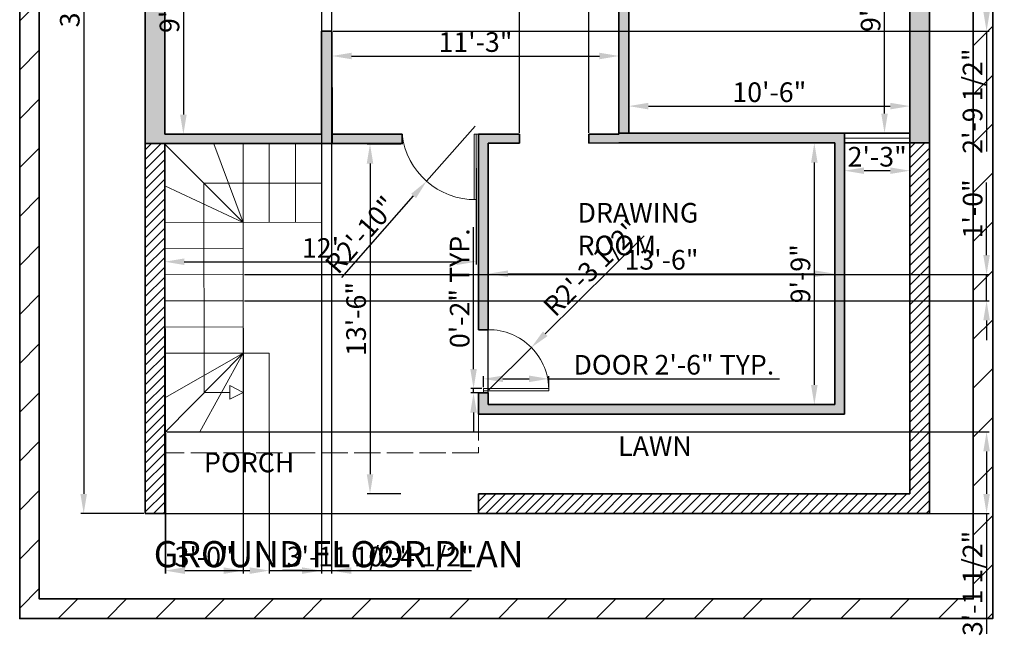
# Model space of a CAD drawing. Units: inches. Extents: x 1130698 to 1131150, y 432269 to 432875.
# Tile 1 of 3: x 1130698 to 1131150, y 432269 to 432551. Entities that reach past the tile are written whole.
import ezdxf

# ---------------------------------------------------------------- set-up
doc = ezdxf.new("R2010")
doc.units = ezdxf.units.IN
doc.linetypes.add('ACAD_ISO02W100', pattern=[15, 12, -3])
for name, color, linetype, lineweight in [('A-ANNO-DIMS', 2, 'Continuous', 18), ('A-ANNO-TEXT', 7, 'Continuous', 25), ('A-ANNO-TTLB', 7, 'Continuous', 35), ('A-AREA-IDEN', 7, 'Continuous', 25), ('A-DOOR', 4, 'Continuous', 18), ('A-FLOR-STRS', 7, 'Continuous', 18), ('A-GLAZ', 4, 'Continuous', 18), ('A-ROOF-OVHD', 8, 'ACAD_ISO02W100', 13), ('A-WALL', 7, 'Continuous', 35)]:
    doc.layers.add(name, color=color, linetype=linetype, lineweight=lineweight)
doc.layers.add('A-ANNO-TTLB-PATT', color=251, linetype='Continuous', lineweight=13, true_color=0x636466)
doc.layers.add('A-WALL-PATT', color=251, linetype='Continuous', lineweight=13, true_color=0x636466)
doc.styles.get("Standard").update_dxf_attribs({"font": 'arial.ttf'})
doc.dimstyles.new('ISO-25', dxfattribs={"dimtxt": 9, "dimasz": 9, "dimexe": 1.25, "dimexo": 0.625, "dimtad": 1, "dimdec": 1, "dimrnd": 9, "dimlunit": 3, "dimtxsty": 'Standard', "dimcen": 2.5, "dimadec": 0, "dimazin": 0, "dimtfac": 1, "dimtdec": 1, "dimtmove": 0, "dimatfit": 3, "dimfxl": 1, "dimarcsym": 0})

# ---------------------------------------------------------------- blocks, each defined once
blk = doc.blocks.new('*D11')
at = {"layer": 'A-ANNO-DIMS', "color": 0, "lineweight": -2, "transparency": 16777216}
for p, q in [((1130977.75, 432499.73), (1130977.75, 432512.76)), ((1130986.75, 432511.51), (1131097.75, 432511.51)), ((1131106.75, 432499.73), (1131106.75, 432512.76))]:
    blk.add_line(p, q, dxfattribs=at)
at = {"layer": 'A-ANNO-DIMS', "color": 0, "transparency": 16777216}
for points in [[(1130986.75, 432513.01), (1130986.75, 432510.01), (1130977.75, 432511.51)], [(1131097.75, 432513.01), (1131097.75, 432510.01), (1131106.75, 432511.51)]]:
    blk.add_solid(points, dxfattribs=at)
at = {"layer": 'Defpoints', "color": 0, "transparency": 16777216}
for p in [(1131106.75, 432511.51), (1130977.75, 432499.11), (1131106.75, 432499.11)]:
    blk.add_point(p, dxfattribs=at)
at = {"layer": 'A-ANNO-DIMS', "color": 0, "transparency": 16777216, "insert": (1131042.25, 432516.73), "char_height": 9, "attachment_point": 5}
blk.add_mtext('10\'-6"', dxfattribs=at)
blk = doc.blocks.new('*D12')
at = {"layer": 'A-ANNO-DIMS', "color": 0, "lineweight": -2, "transparency": 16777216}
for p, q in [((1131106.12, 432619.11), (1131093.87, 432619.11)), ((1131095.12, 432508.11), (1131095.12, 432610.11)), ((1131106.12, 432499.11), (1131093.87, 432499.11))]:
    blk.add_line(p, q, dxfattribs=at)
at = {"layer": 'A-ANNO-DIMS', "color": 0, "transparency": 16777216}
for points in [[(1131093.62, 432610.11), (1131096.62, 432610.11), (1131095.12, 432619.11)], [(1131093.62, 432508.11), (1131096.62, 432508.11), (1131095.12, 432499.11)]]:
    blk.add_solid(points, dxfattribs=at)
at = {"layer": 'Defpoints', "color": 0, "transparency": 16777216}
for p in [(1131095.12, 432619.11), (1131106.75, 432619.11), (1131106.75, 432499.11)]:
    blk.add_point(p, dxfattribs=at)
at = {"layer": 'A-ANNO-DIMS', "color": 0, "transparency": 16777216, "insert": (1131089.9, 432559.11), "char_height": 9, "attachment_point": 5, "rotation": 90}
blk.add_mtext('9\'-9"', dxfattribs=at)
blk = doc.blocks.new('*D13')
at = {"layer": 'A-ANNO-DIMS', "color": 0, "lineweight": -2, "transparency": 16777216}
for p, q in [((1130765.37, 432618.61), (1130774.58, 432618.61)), ((1130773.33, 432609.61), (1130773.33, 432507.61)), ((1130765.37, 432498.61), (1130774.58, 432498.61))]:
    blk.add_line(p, q, dxfattribs=at)
at = {"layer": 'A-ANNO-DIMS', "color": 0, "transparency": 16777216}
for points in [[(1130771.83, 432609.61), (1130774.83, 432609.61), (1130773.33, 432618.61)], [(1130771.83, 432507.61), (1130774.83, 432507.61), (1130773.33, 432498.61)]]:
    blk.add_solid(points, dxfattribs=at)
at = {"layer": 'Defpoints', "color": 0, "transparency": 16777216}
for p in [(1130764.75, 432618.61), (1130764.75, 432498.61), (1130773.33, 432498.61)]:
    blk.add_point(p, dxfattribs=at)
at = {"layer": 'A-ANNO-DIMS', "color": 0, "transparency": 16777216, "insert": (1130768.11, 432558.61), "char_height": 9, "attachment_point": 5, "rotation": 90}
blk.add_mtext('9\'-9"', dxfattribs=at)
blk = doc.blocks.new('*D15')
at = {"layer": 'A-ANNO-DIMS', "color": 0, "lineweight": -2, "transparency": 16777216}
for p, q in [((1130841.53, 432499.23), (1130841.53, 432535.75)), ((1130850.53, 432534.5), (1130964.25, 432534.5)), ((1130973.25, 432499.73), (1130973.25, 432535.75))]:
    blk.add_line(p, q, dxfattribs=at)
at = {"layer": 'A-ANNO-DIMS', "color": 0, "transparency": 16777216}
for points in [[(1130850.53, 432536), (1130850.53, 432533), (1130841.53, 432534.5)], [(1130964.25, 432536), (1130964.25, 432533), (1130973.25, 432534.5)]]:
    blk.add_solid(points, dxfattribs=at)
at = {"layer": 'Defpoints', "color": 0, "transparency": 16777216}
for p in [(1130973.25, 432534.5), (1130841.53, 432498.61), (1130973.25, 432499.11)]:
    blk.add_point(p, dxfattribs=at)
at = {"layer": 'A-ANNO-DIMS', "color": 0, "transparency": 16777216, "insert": (1130907.39, 432539.73), "char_height": 9, "attachment_point": 5}
blk.add_mtext('11\'-3"', dxfattribs=at)
blk = doc.blocks.new('*D16')
at = {"layer": 'A-ANNO-DIMS', "color": 0, "lineweight": -2, "transparency": 16777216}
for p, q in [((1131071.62, 432494.61), (1131061.65, 432494.61)), ((1131062.9, 432485.61), (1131062.9, 432383.61)), ((1131071.62, 432374.61), (1131061.65, 432374.61))]:
    blk.add_line(p, q, dxfattribs=at)
at = {"layer": 'A-ANNO-DIMS', "color": 0, "transparency": 16777216}
for points in [[(1131061.4, 432485.61), (1131064.4, 432485.61), (1131062.9, 432494.61)], [(1131061.4, 432383.61), (1131064.4, 432383.61), (1131062.9, 432374.61)]]:
    blk.add_solid(points, dxfattribs=at)
at = {"layer": 'Defpoints', "color": 0, "transparency": 16777216}
for p in [(1131072.25, 432494.61), (1131062.9, 432374.61), (1131072.25, 432374.61)]:
    blk.add_point(p, dxfattribs=at)
at = {"layer": 'A-ANNO-DIMS', "color": 0, "transparency": 16777216, "insert": (1131057.68, 432434.61), "char_height": 9, "attachment_point": 5, "rotation": 90}
blk.add_mtext('9\'-9"', dxfattribs=at)
blk = doc.blocks.new('*D17')
at = {"layer": 'A-ANNO-DIMS', "color": 0, "lineweight": -2, "transparency": 16777216}
for p, q in [((1130913.25, 432375.23), (1130913.25, 432435.86)), ((1130922.25, 432434.61), (1131063.25, 432434.61)), ((1131072.25, 432375.23), (1131072.25, 432435.86))]:
    blk.add_line(p, q, dxfattribs=at)
at = {"layer": 'A-ANNO-DIMS', "color": 0, "transparency": 16777216}
for points in [[(1130922.25, 432436.11), (1130922.25, 432433.11), (1130913.25, 432434.61)], [(1131063.25, 432436.11), (1131063.25, 432433.11), (1131072.25, 432434.61)]]:
    blk.add_solid(points, dxfattribs=at)
at = {"layer": 'Defpoints', "color": 0, "transparency": 16777216}
for p in [(1131072.25, 432434.61), (1130913.25, 432374.61), (1131072.25, 432374.61)]:
    blk.add_point(p, dxfattribs=at)
at = {"layer": 'A-ANNO-DIMS', "color": 0, "transparency": 16777216, "insert": (1130992.75, 432439.83), "char_height": 9, "attachment_point": 5}
blk.add_mtext('13\'-6"', dxfattribs=at)
blk = doc.blocks.new('*D18')
at = {"layer": 'A-ANNO-DIMS', "color": 0, "lineweight": -2, "transparency": 16777216}
for p, q in [((1130873.07, 432494.11), (1130857.73, 432494.11)), ((1130858.98, 432485.11), (1130858.98, 432342.61)), ((1130873.07, 432333.61), (1130857.73, 432333.61))]:
    blk.add_line(p, q, dxfattribs=at)
at = {"layer": 'A-ANNO-DIMS', "color": 0, "transparency": 16777216}
for points in [[(1130857.48, 432485.11), (1130860.48, 432485.11), (1130858.98, 432494.11)], [(1130857.48, 432342.61), (1130860.48, 432342.61), (1130858.98, 432333.61)]]:
    blk.add_solid(points, dxfattribs=at)
at = {"layer": 'Defpoints', "color": 0, "transparency": 16777216}
for p in [(1130873.7, 432494.11), (1130858.98, 432333.61), (1130873.7, 432333.61)]:
    blk.add_point(p, dxfattribs=at)
at = {"layer": 'A-ANNO-DIMS', "color": 0, "transparency": 16777216, "insert": (1130853.76, 432413.86), "char_height": 9, "attachment_point": 5, "rotation": 90}
blk.add_mtext('13\'-6"', dxfattribs=at)
blk = doc.blocks.new('*D19')
at = {"layer": 'A-ANNO-DIMS', "color": 0, "lineweight": -2, "transparency": 16777216}
for p, q in [((1130764.75, 432493.48), (1130764.75, 432438.87)), ((1130907.75, 432482.98), (1130907.75, 432438.87)), ((1130773.75, 432440.12), (1130898.75, 432440.12))]:
    blk.add_line(p, q, dxfattribs=at)
at = {"layer": 'A-ANNO-DIMS', "color": 0, "transparency": 16777216}
for points in [[(1130773.75, 432441.62), (1130773.75, 432438.62), (1130764.75, 432440.12)], [(1130898.75, 432441.62), (1130898.75, 432438.62), (1130907.75, 432440.12)]]:
    blk.add_solid(points, dxfattribs=at)
at = {"layer": 'Defpoints', "color": 0, "transparency": 16777216}
for p in [(1130764.75, 432494.11), (1130907.75, 432483.61), (1130907.75, 432440.12)]:
    blk.add_point(p, dxfattribs=at)
at = {"layer": 'A-ANNO-DIMS', "color": 0, "transparency": 16777216, "insert": (1130836.25, 432445.26), "char_height": 9, "attachment_point": 5}
blk.add_mtext("12'", dxfattribs=at)
blk = doc.blocks.new('*D21')
at = {"layer": 'A-ANNO-DIMS', "color": 0, "lineweight": -2, "transparency": 16777216}
for p, q in [((1130755.12, 432804.61), (1130726.33, 432804.61)), ((1130727.58, 432795.61), (1130727.58, 432333.61)), ((1130755.12, 432324.61), (1130726.33, 432324.61))]:
    blk.add_line(p, q, dxfattribs=at)
at = {"layer": 'A-ANNO-DIMS', "color": 0, "transparency": 16777216}
for points in [[(1130726.08, 432795.61), (1130729.08, 432795.61), (1130727.58, 432804.61)], [(1130726.08, 432333.61), (1130729.08, 432333.61), (1130727.58, 432324.61)]]:
    blk.add_solid(points, dxfattribs=at)
at = {"layer": 'Defpoints', "color": 0, "transparency": 16777216}
for p in [(1130755.75, 432804.61), (1130727.58, 432324.61), (1130755.75, 432324.61)]:
    blk.add_point(p, dxfattribs=at)
at = {"layer": 'A-ANNO-DIMS', "color": 0, "transparency": 16777216, "insert": (1130722.35, 432564.61), "char_height": 9, "attachment_point": 5, "rotation": 90}
blk.add_mtext('39\'-9"', dxfattribs=at)
blk = doc.blocks.new('*D22')
at = {"layer": 'A-ANNO-DIMS', "color": 0, "lineweight": -2, "transparency": 16777216}
for p, q in [((1131076.75, 432493.98), (1131076.75, 432480.63)), ((1131106.75, 432493.98), (1131106.75, 432480.63)), ((1131097.75, 432481.88), (1131085.75, 432481.88))]:
    blk.add_line(p, q, dxfattribs=at)
at = {"layer": 'A-ANNO-DIMS', "color": 0, "transparency": 16777216}
for points in [[(1131085.75, 432483.38), (1131085.75, 432480.38), (1131076.75, 432481.88)], [(1131097.75, 432483.38), (1131097.75, 432480.38), (1131106.75, 432481.88)]]:
    blk.add_solid(points, dxfattribs=at)
at = {"layer": 'Defpoints', "color": 0, "transparency": 16777216}
for p in [(1131076.75, 432494.61), (1131106.75, 432494.61), (1131076.75, 432481.88)]:
    blk.add_point(p, dxfattribs=at)
at = {"layer": 'A-ANNO-DIMS', "color": 0, "transparency": 16777216, "insert": (1131091.75, 432487.11), "char_height": 9, "attachment_point": 5}
blk.add_mtext('2\'-3"', dxfattribs=at)
blk = doc.blocks.new('DOOR-LEAF-30IN')
for p, q in [((30, 2), (0, 2)), ((0, 2), (0, 1)), ((0, 0), (0, 1)), ((0, 1), (30, 1)), ((30, 1), (30, 2))]:
    blk.add_line(p, q)
blk = doc.blocks.new('*D28')
at = {"layer": 'A-ANNO-DIMS', "color": 0, "lineweight": -2, "transparency": 16777216}
for p, q in [((1130911, 432382.53), (1130911, 432387.65)), ((1130941, 432382.53), (1130941, 432387.65)), ((1130920, 432386.4), (1130932, 432386.4)), ((1130941, 432386.4), (1131046.87, 432386.4))]:
    blk.add_line(p, q, dxfattribs=at)
at = {"layer": 'A-ANNO-DIMS', "color": 0, "transparency": 16777216}
for points in [[(1130920, 432387.9), (1130920, 432384.9), (1130911, 432386.4)], [(1130932, 432387.9), (1130932, 432384.9), (1130941, 432386.4)]]:
    blk.add_solid(points, dxfattribs=at)
at = {"layer": 'Defpoints', "color": 0, "transparency": 16777216}
for p in [(1130941, 432386.4), (1130911, 432381.9), (1130941, 432381.9)]:
    blk.add_point(p, dxfattribs=at)
at = {"layer": 'A-ANNO-DIMS', "color": 0, "transparency": 16777216, "insert": (1130998.43, 432391.69), "char_height": 9, "attachment_point": 5}
blk.add_mtext('DOOR 2\'-6" TYP.', dxfattribs=at)
blk = doc.blocks.new('*D29')
at = {"layer": 'A-ANNO-DIMS', "color": 0, "lineweight": -2, "transparency": 16777216}
for p, q in [((1130906.5, 432390.9), (1130906.5, 432456.01)), ((1130910.37, 432381.9), (1130905.25, 432381.9)), ((1130910.37, 432379.9), (1130905.25, 432379.9)), ((1130906.5, 432379.9), (1130906.5, 432381.9)), ((1130906.5, 432370.9), (1130906.5, 432361.9))]:
    blk.add_line(p, q, dxfattribs=at)
at = {"layer": 'A-ANNO-DIMS', "color": 0, "transparency": 16777216}
for points in [[(1130905, 432390.9), (1130908, 432390.9), (1130906.5, 432381.9)], [(1130905, 432370.9), (1130908, 432370.9), (1130906.5, 432379.9)]]:
    blk.add_solid(points, dxfattribs=at)
at = {"layer": 'Defpoints', "color": 0, "transparency": 16777216}
for p in [(1130906.5, 432381.9), (1130911, 432381.9), (1130911, 432379.9)]:
    blk.add_point(p, dxfattribs=at)
at = {"layer": 'A-ANNO-DIMS', "color": 0, "transparency": 16777216, "insert": (1130901.28, 432427.96), "char_height": 9, "attachment_point": 5, "rotation": 90}
blk.add_mtext('0\'-2" TYP.', dxfattribs=at)
blk = doc.blocks.new('*D32')
at = {"layer": 'A-ANNO-DIMS', "color": 0, "lineweight": -2, "transparency": 16777216}
for p, q in [((1130765.06, 432361.48), (1130765.06, 432297.16)), ((1130812.75, 432361.6), (1130812.75, 432297.16)), ((1130774.06, 432298.41), (1130803.75, 432298.41)), ((1130812.75, 432298.41), (1130874.88, 432298.41))]:
    blk.add_line(p, q, dxfattribs=at)
at = {"layer": 'A-ANNO-DIMS', "color": 0, "transparency": 16777216}
for points in [[(1130774.06, 432299.91), (1130774.06, 432296.91), (1130765.06, 432298.41)], [(1130803.75, 432299.91), (1130803.75, 432296.91), (1130812.75, 432298.41)]]:
    blk.add_solid(points, dxfattribs=at)
at = {"layer": 'Defpoints', "color": 0, "transparency": 16777216}
for p in [(1130765.06, 432362.11), (1130812.75, 432362.22), (1130812.75, 432298.41)]:
    blk.add_point(p, dxfattribs=at)
at = {"layer": 'A-ANNO-DIMS', "color": 0, "transparency": 16777216, "insert": (1130848.31, 432303.69), "char_height": 9, "attachment_point": 5}
blk.add_mtext('3\'-11 1/2"', dxfattribs=at)
blk = doc.blocks.new('*D33')
at = {"layer": 'A-ANNO-DIMS', "color": 0, "lineweight": -2, "transparency": 16777216}
for p, q in [((1131141.95, 432443.19), (1131141.95, 432476.52)), ((1130801.37, 432434.19), (1131143.2, 432434.19)), ((1131141.95, 432422.19), (1131141.95, 432434.19)), ((1130801.37, 432422.19), (1131143.2, 432422.19)), ((1131141.95, 432413.19), (1131141.95, 432404.19))]:
    blk.add_line(p, q, dxfattribs=at)
at = {"layer": 'A-ANNO-DIMS', "color": 0, "transparency": 16777216}
for points in [[(1131140.45, 432443.19), (1131143.45, 432443.19), (1131141.95, 432434.19)], [(1131140.45, 432413.19), (1131143.45, 432413.19), (1131141.95, 432422.19)]]:
    blk.add_solid(points, dxfattribs=at)
at = {"layer": 'Defpoints', "color": 0, "transparency": 16777216}
for p in [(1130800.75, 432434.19), (1131141.95, 432434.19), (1130800.75, 432422.19)]:
    blk.add_point(p, dxfattribs=at)
at = {"layer": 'A-ANNO-DIMS', "color": 0, "transparency": 16777216, "insert": (1131136.73, 432464.36), "char_height": 9, "attachment_point": 5, "rotation": 90}
blk.add_mtext('1\'-0"', dxfattribs=at)
blk = doc.blocks.new('*D34')
at = {"layer": 'A-ANNO-DIMS', "color": 0, "lineweight": -2, "transparency": 16777216}
for p, q in [((1130764.95, 432409.48), (1130764.95, 432297.16)), ((1130800.75, 432409.57), (1130800.75, 432297.16)), ((1130773.95, 432298.41), (1130791.75, 432298.41))]:
    blk.add_line(p, q, dxfattribs=at)
at = {"layer": 'A-ANNO-DIMS', "color": 0, "transparency": 16777216}
for points in [[(1130773.95, 432299.91), (1130773.95, 432296.91), (1130764.95, 432298.41)], [(1130791.75, 432299.91), (1130791.75, 432296.91), (1130800.75, 432298.41)]]:
    blk.add_solid(points, dxfattribs=at)
at = {"layer": 'Defpoints', "color": 0, "transparency": 16777216}
for p in [(1130764.95, 432410.11), (1130800.75, 432410.19), (1130800.75, 432298.41)]:
    blk.add_point(p, dxfattribs=at)
at = {"layer": 'A-ANNO-DIMS', "color": 0, "transparency": 16777216, "insert": (1130782.85, 432303.63), "char_height": 9, "attachment_point": 5}
blk.add_mtext('3\'-0"', dxfattribs=at)
blk = doc.blocks.new('*D35')
at = {"layer": 'A-ANNO-DIMS', "color": 0, "lineweight": -2, "transparency": 16777216}
for p, q in [((1130765.69, 432362.11), (1131143.2, 432362.11)), ((1131141.95, 432353.11), (1131141.95, 432333.61)), ((1130765.37, 432324.61), (1131143.2, 432324.61)), ((1131141.95, 432324.61), (1131141.95, 432269.47))]:
    blk.add_line(p, q, dxfattribs=at)
at = {"layer": 'A-ANNO-DIMS', "color": 0, "transparency": 16777216}
for points in [[(1131140.45, 432353.11), (1131143.45, 432353.11), (1131141.95, 432362.11)], [(1131140.45, 432333.61), (1131143.45, 432333.61), (1131141.95, 432324.61)]]:
    blk.add_solid(points, dxfattribs=at)
at = {"layer": 'Defpoints', "color": 0, "transparency": 16777216}
for p in [(1130765.06, 432362.11), (1130764.75, 432324.61), (1131141.95, 432324.61)]:
    blk.add_point(p, dxfattribs=at)
at = {"layer": 'A-ANNO-DIMS', "color": 0, "transparency": 16777216, "insert": (1131136.66, 432292.54), "char_height": 9, "attachment_point": 5, "rotation": 90}
blk.add_mtext('3\'-1 1/2"', dxfattribs=at)
blk = doc.blocks.new('*D36')
at = {"layer": 'A-ANNO-DIMS', "color": 0, "lineweight": -2, "transparency": 16777216}
for p, q in [((1130841.96, 432579.47), (1131143.2, 432579.47)), ((1131141.95, 432570.47), (1131141.95, 432554.94)), ((1130842.05, 432545.94), (1131143.2, 432545.94)), ((1131141.95, 432545.94), (1131141.95, 432490.64))]:
    blk.add_line(p, q, dxfattribs=at)
at = {"layer": 'A-ANNO-DIMS', "color": 0, "transparency": 16777216}
for points in [[(1131140.45, 432570.47), (1131143.45, 432570.47), (1131141.95, 432579.47)], [(1131140.45, 432554.94), (1131143.45, 432554.94), (1131141.95, 432545.94)]]:
    blk.add_solid(points, dxfattribs=at)
at = {"layer": 'Defpoints', "color": 0, "transparency": 16777216}
for p in [(1130841.34, 432579.47), (1130841.42, 432545.94), (1131141.95, 432545.94)]:
    blk.add_point(p, dxfattribs=at)
at = {"layer": 'A-ANNO-DIMS', "color": 0, "transparency": 16777216, "insert": (1131136.67, 432513.79), "char_height": 9, "attachment_point": 5, "rotation": 90}
blk.add_mtext('2\'-9 1/2"', dxfattribs=at)
blk = doc.blocks.new('*D38')
at = {"layer": 'A-ANNO-DIMS', "color": 0, "lineweight": -2, "transparency": 16777216}
for p, q in [((1130927.61, 432499.23), (1130927.61, 432832.06)), ((1130936.61, 432830.81), (1130950.44, 432830.81)), ((1130959.44, 432499.23), (1130959.44, 432832.06))]:
    blk.add_line(p, q, dxfattribs=at)
at = {"layer": 'A-ANNO-DIMS', "color": 0, "transparency": 16777216}
for points in [[(1130936.61, 432832.31), (1130936.61, 432829.31), (1130927.61, 432830.81)], [(1130950.44, 432832.31), (1130950.44, 432829.31), (1130959.44, 432830.81)]]:
    blk.add_solid(points, dxfattribs=at)
at = {"layer": 'Defpoints', "color": 0, "transparency": 16777216}
for p in [(1130959.44, 432830.81), (1130927.61, 432498.61), (1130959.44, 432498.61)]:
    blk.add_point(p, dxfattribs=at)
at = {"layer": 'A-ANNO-DIMS', "color": 0, "transparency": 16777216, "insert": (1130943.52, 432836.03), "char_height": 9, "attachment_point": 5}
blk.add_mtext('2\'-8"', dxfattribs=at)
blk = doc.blocks.new('*D39')
at = {"layer": 'A-ANNO-DIMS', "color": 0, "lineweight": -2, "transparency": 16777216}
for p, q in [((1130950.44, 432830.81), (1130941.44, 432830.81)), ((1130959.44, 432499.23), (1130959.44, 432832.06)), ((1130959.44, 432830.81), (1130973.25, 432830.81)), ((1130973.25, 432499.73), (1130973.25, 432832.06)), ((1130982.25, 432830.81), (1131015.57, 432830.81))]:
    blk.add_line(p, q, dxfattribs=at)
at = {"layer": 'A-ANNO-DIMS', "color": 0, "transparency": 16777216}
for points in [[(1130950.44, 432832.31), (1130950.44, 432829.31), (1130959.44, 432830.81)], [(1130982.25, 432832.31), (1130982.25, 432829.31), (1130973.25, 432830.81)]]:
    blk.add_solid(points, dxfattribs=at)
at = {"layer": 'Defpoints', "color": 0, "transparency": 16777216}
for p in [(1130973.25, 432830.81), (1130959.44, 432498.61), (1130973.25, 432499.11)]:
    blk.add_point(p, dxfattribs=at)
at = {"layer": 'A-ANNO-DIMS', "color": 0, "transparency": 16777216, "insert": (1131003.41, 432835.95), "char_height": 9, "attachment_point": 5}
blk.add_mtext('1\'-2"', dxfattribs=at)
blk = doc.blocks.new('*D41')
at = {"layer": 'A-ANNO-DIMS', "color": 0, "lineweight": -2, "transparency": 16777216}
for p, q in [((1130836.75, 432578.84), (1130836.75, 432297.16)), ((1130841.34, 432578.84), (1130841.34, 432297.16)), ((1130827.75, 432298.41), (1130818.75, 432298.41)), ((1130836.75, 432298.41), (1130841.34, 432298.41)), ((1130850.34, 432298.41), (1130905.49, 432298.41))]:
    blk.add_line(p, q, dxfattribs=at)
at = {"layer": 'A-ANNO-DIMS', "color": 0, "transparency": 16777216}
for points in [[(1130827.75, 432299.91), (1130827.75, 432296.91), (1130836.75, 432298.41)], [(1130850.34, 432299.91), (1130850.34, 432296.91), (1130841.34, 432298.41)]]:
    blk.add_solid(points, dxfattribs=at)
at = {"layer": 'Defpoints', "color": 0, "transparency": 16777216}
for p in [(1130836.75, 432579.47), (1130841.34, 432579.47), (1130841.34, 432298.41)]:
    blk.add_point(p, dxfattribs=at)
at = {"layer": 'A-ANNO-DIMS', "color": 0, "transparency": 16777216, "insert": (1130882.41, 432303.68), "char_height": 9, "attachment_point": 5}
blk.add_mtext('0\'-4 1/2"', dxfattribs=at)
blk = doc.blocks.new('*D43')
at = {"layer": 'A-ANNO-DIMS', "color": 0, "lineweight": -2, "transparency": 16777216}
for p, q in [((1130907.25, 432502.36), (1130884.93, 432477.03)), ((1130846.07, 432432.93), (1130878.98, 432470.28))]:
    blk.add_line(p, q, dxfattribs=at)
at = {"layer": 'A-ANNO-DIMS', "color": 0, "transparency": 16777216}
blk.add_solid([(1130877.85, 432471.27), (1130880.1, 432469.29), (1130884.93, 432477.03)], dxfattribs=at)
at = {"layer": 'Defpoints', "color": 0, "transparency": 16777216}
for p in [(1130907.25, 432502.36), (1130884.93, 432477.03)]:
    blk.add_point(p, dxfattribs=at)
at = {"layer": 'A-ANNO-DIMS', "color": 0, "transparency": 16777216, "insert": (1130855.63, 432451.68), "char_height": 9, "attachment_point": 5, "rotation": 48.6159}
blk.add_mtext('R2\'-10"', dxfattribs=at)
blk = doc.blocks.new('*D47')
at = {"layer": 'A-ANNO-DIMS', "color": 0, "lineweight": -2, "transparency": 16777216}
for p, q in [((1130984.74, 432451.96), (1130939.43, 432407.11)), ((1130913.47, 432381.4), (1130933.03, 432400.78))]:
    blk.add_line(p, q, dxfattribs=at)
at = {"layer": 'A-ANNO-DIMS', "color": 0, "transparency": 16777216}
blk.add_solid([(1130938.37, 432408.17), (1130940.49, 432406.04), (1130933.03, 432400.78)], dxfattribs=at)
at = {"layer": 'Defpoints', "color": 0, "transparency": 16777216}
for p in [(1130933.03, 432400.78), (1130913.47, 432381.4)]:
    blk.add_point(p, dxfattribs=at)
at = {"layer": 'A-ANNO-DIMS', "color": 0, "transparency": 16777216, "insert": (1130961.57, 432436.45), "char_height": 9, "attachment_point": 5, "rotation": 44.7103}
blk.add_mtext('R2\'-3 1/2"', dxfattribs=at)

msp = doc.modelspace()

# ---------------------------------------------------------------- hatches: boundary and pattern name
at = {"layer": 'A-ANNO-TTLB-PATT'}
h = msp.add_hatch(dxfattribs=at)
h.set_pattern_fill('ANSI31', color=256, scale=5)
h.paths.add_polyline_path([(1131144.8, 432864.01), (1130698.2, 432864.01), (1130698.2, 432276.41), (1131144.8, 432276.41)])
h.paths.add_polyline_path([(1130707.2, 432855.01), (1131135.8, 432855.01), (1131135.8, 432285.41), (1130707.2, 432285.41)], flags=16)
h.paths.add_polyline_path([(1130755.75, 432804.61), (1131115.75, 432804.61), (1131115.75, 432324.61), (1130908.75, 432324.61), (1130908.75, 432333.61), (1131106.75, 432333.61), (1131106.75, 432494.61), (1131076.75, 432494.61), (1131076.75, 432370.11), (1130908.75, 432370.11), (1130908.75, 432352.4), (1130764.75, 432352.4), (1130764.75, 432333.61), (1130764.75, 432324.61), (1130755.75, 432324.61)], flags=0)
h.paths.add_polyline_path([(1130764.75, 432795.61), (1130836.75, 432795.61), (1130836.75, 432747.61), (1130841.25, 432747.61), (1130841.25, 432795.61), (1130973.25, 432795.61), (1130973.25, 432747.61), (1130977.75, 432747.61), (1130977.75, 432795.61), (1130986.75, 432795.61), (1131106.75, 432795.61), (1131106.75, 432499.11), (1130973.25, 432499.11), (1130973.25, 432498.61), (1130959.44, 432498.61), (1130959.45, 432494.57), (1130973.25, 432494.61), (1131072.25, 432494.61), (1131072.25, 432374.61), (1130913.25, 432374.61), (1130913.25, 432379.9), (1130911, 432379.9), (1130911, 432380.9), (1130911, 432381.9), (1130941, 432381.9, 0.411251), (1130913.25, 432408.94), (1130908.75, 432408.94), (1130908.75, 432498.61), (1130907.75, 432498.61), (1130907.75, 432468.61, -0.386197), (1130873.7, 432498.61), (1130873.7, 432494.37), (1130841.54, 432494.37), (1130841.42, 432545.94), (1130836.75, 432545.94), (1130836.75, 432498.61), (1130764.75, 432498.61), (1130764.75, 432618.61), (1130836.75, 432618.61), (1130836.75, 432579.47), (1130841.34, 432579.47), (1130841.25, 432618.61), (1130874.63, 432618.61), (1130874.63, 432620.86, -0.017137), (1130874.63, 432623.09), (1130874.63, 432623.11), (1130764.75, 432623.11), (1130764.75, 432738.61), (1130764.75, 432743.11), (1130764.75, 432747.61)], flags=0)
h.paths.add_polyline_path([(1130765.75, 432769.36, -0.376584), (1130794.09, 432745.36), (1130794.09, 432743.11), (1130908.75, 432743.11), (1130908.75, 432618.61), (1130913.25, 432618.61), (1130913.25, 432743.11), (1130973.25, 432743.11), (1130973.25, 432664.11), (1130938.73, 432664.11), (1130938.73, 432659.61), (1130977.75, 432659.61, -0.392039), (1131009.25, 432624.61), (1130973.25, 432624.61), (1130973.25, 432623.61), (1130973.25, 432619.11), (1130973.25, 432618.11), (1131009.25, 432618.11, -0.432961), (1130975.5, 432585.44), (1130977.75, 432585.44), (1130977.75, 432585.41, 0.403315), (1131009.25, 432617.11), (1130973.25, 432617.11), (1130973.25, 432618.11), (1130973.25, 432619.11), (1130973.25, 432623.61), (1130973.25, 432624.61), (1130973.25, 432625.61), (1131009.25, 432625.61, 0.383736), (1130977.75, 432659.61), (1130938.73, 432659.61, 0.405522), (1130915.25, 432683.38), (1130915.25, 432659.38), (1130914.25, 432659.38), (1130913.25, 432659.38), (1130913.25, 432618.61), (1130908.75, 432618.61), (1130907.75, 432618.61), (1130906.75, 432618.61), (1130906.75, 432654.61), (1130907.75, 432654.61), (1130907.75, 432618.61), (1130908.75, 432618.61), (1130908.75, 432743.11), (1130794.09, 432743.11), (1130794.09, 432745.36, 0.366478), (1130766.75, 432769.36), (1130766.75, 432745.36), (1130765.75, 432745.36)], flags=0)
h.paths.add_polyline_path([(1130782.75, 432476.15), (1130836.75, 432476.19), (1130836.75, 432458.28), (1130800.75, 432458.19), (1130800.75, 432398.19), (1130812.75, 432398.22), (1130812.75, 432362.22), (1130765.06, 432362.11), (1130782.9, 432380.15)], flags=0)
h.paths.add_polyline_path([(1130794.59, 432383.39), (1130800.75, 432380.15), (1130794.59, 432377.08)], flags=0)
h.paths.add_polyline_path([(1130793.86, 432783.91), (1130807.75, 432783.91), (1130807.75, 432802.46), (1130793.86, 432802.46)], flags=8)
h.paths.add_polyline_path([(1130833.23, 432764.87), (1130833.23, 432778.77), (1130814.69, 432778.77), (1130814.69, 432764.87)], flags=8)
h.paths.add_polyline_path([(1130888.59, 432778.49), (1130925.12, 432778.49), (1130925.12, 432797.04), (1130888.59, 432797.04)], flags=8)
h.paths.add_polyline_path([(1130854.91, 432764.87), (1130854.91, 432778.77), (1130836.36, 432778.77), (1130836.36, 432764.87)], flags=8)
h.paths.add_polyline_path([(1131023.59, 432772.28), (1131060.12, 432772.28), (1131060.12, 432790.83), (1131023.59, 432790.83)], flags=8)
h.paths.add_polyline_path([(1130825.91, 432723.63), (1130846.8, 432723.63), (1130846.8, 432742.18), (1130825.91, 432742.18)], flags=8)
h.paths.add_polyline_path([(1130901.54, 432668.37), (1130901.54, 432697.91), (1130882.99, 432697.91), (1130882.99, 432668.37)], flags=8)
h.paths.add_polyline_path([(1130928.51, 432726.62), (1130958.05, 432726.62), (1130958.05, 432745.17), (1130928.51, 432745.17)], flags=8)
h.paths.add_polyline_path([(1130972.51, 432688.9), (1130972.51, 432718.43), (1130953.97, 432718.43), (1130953.97, 432688.9)], flags=8)
h.paths.add_polyline_path([(1130925.33, 432811.35), (1130946.22, 432811.35), (1130946.22, 432829.9), (1130925.33, 432829.9)], flags=8)
h.paths.add_polyline_path([(1130731.71, 432554.38), (1130731.71, 432575.26), (1130713.17, 432575.26), (1130713.17, 432554.38)], flags=8)
h.paths.add_polyline_path([(1130755.82, 432293.19), (1130947.18, 432293.19), (1130947.18, 432317.92), (1130755.82, 432317.92)], flags=8)
h.paths.add_polyline_path([(1130779.57, 432338.43), (1130829.48, 432338.43), (1130829.48, 432356.98), (1130779.57, 432356.98)], flags=8)
h.paths.add_polyline_path([(1130969.67, 432346.11), (1131010.5, 432346.11), (1131010.5, 432364.66), (1130969.67, 432364.66)], flags=8)
h.paths.add_polyline_path([(1130950.99, 432437.85), (1131016.28, 432437.85), (1131016.28, 432471.55), (1130950.99, 432471.55)], flags=8)
h.paths.add_polyline_path([(1130780.08, 432552.69), (1130839.77, 432552.69), (1130839.77, 432571.24), (1130780.08, 432571.24)], flags=8)
h.paths.add_polyline_path([(1130996.81, 432568.37), (1131080.25, 432568.37), (1131080.25, 432586.92), (1130996.81, 432586.92)], flags=8)
h.paths.add_polyline_path([(1130877.83, 432553.22), (1130935.44, 432553.22), (1130935.44, 432586.93), (1130877.83, 432586.93)], flags=8)
h.paths.add_polyline_path([(1130919.84, 432705.86), (1130945.29, 432705.86), (1130945.29, 432724.41), (1130919.84, 432724.41)], flags=8)
h.paths.add_polyline_path([(1131004.1, 432697.07), (1131077.07, 432697.07), (1131077.07, 432730.77), (1131004.1, 432730.77)], flags=8)
h.paths.add_polyline_path([(1130782.53, 432767.61), (1130807.98, 432767.61), (1130807.98, 432786.15), (1130782.53, 432786.15)], flags=8)
h.paths.add_polyline_path([(1130874.11, 432757.47), (1130904.45, 432757.47), (1130904.45, 432776.02), (1130874.11, 432776.02)], flags=8)
h.paths.add_polyline_path([(1130785.78, 432691.47), (1130858.74, 432691.47), (1130858.74, 432710.01), (1130785.78, 432710.01)], flags=8)
at = {"layer": 'A-WALL-PATT'}
h = msp.add_hatch(color=256, dxfattribs=at)
h.dxf.hatch_style = 1
h.paths.add_polyline_path([(1130764.75, 432738.61), (1130764.75, 432743.11), (1130764.75, 432747.61), (1130764.75, 432795.61), (1130836.75, 432795.61), (1130836.75, 432747.61), (1130841.25, 432747.61), (1130841.25, 432795.61), (1130973.25, 432795.61), (1130973.25, 432747.61), (1130977.75, 432747.61), (1130977.75, 432795.61), (1130986.75, 432795.61), (1131106.75, 432795.61), (1131106.75, 432499.11), (1131106.75, 432494.61), (1131115.75, 432494.61), (1131115.75, 432804.61), (1130755.75, 432804.61), (1130755.75, 432494.37), (1130841.54, 432494.37), (1130841.42, 432545.94), (1130836.75, 432545.94), (1130836.75, 432498.61), (1130764.75, 432498.61), (1130764.75, 432618.61), (1130836.75, 432618.61), (1130836.75, 432579.47), (1130841.34, 432579.47), (1130841.25, 432618.61), (1130874.63, 432618.61), (1130874.63, 432623.11), (1130764.75, 432623.11)])
h.paths.add_polyline_path([(1131106.75, 432623.61), (1130973.25, 432623.61), (1130973.25, 432619.11), (1131106.75, 432619.11)], flags=17)
h.paths.add_polyline_path([(1130913.25, 432743.11), (1130973.25, 432743.11), (1130973.25, 432664.11), (1130938.73, 432664.11), (1130938.73, 432659.61), (1130977.75, 432659.61), (1130977.75, 432743.11), (1130977.75, 432747.61), (1130973.25, 432747.61), (1130794.09, 432747.61), (1130794.09, 432743.11), (1130908.75, 432743.11), (1130908.75, 432618.61), (1130913.25, 432618.61)], flags=17)
h.paths.add_polyline_path([(1131076.75, 432499.11), (1130973.25, 432499.11), (1130973.25, 432498.61), (1130959.44, 432498.61), (1130959.45, 432494.57), (1130973.25, 432494.61), (1131072.25, 432494.61), (1131072.25, 432374.61), (1130913.25, 432374.61), (1130913.25, 432379.9), (1130908.75, 432379.9), (1130908.75, 432370.11), (1131076.75, 432370.11)])
h.paths.add_polyline_path([(1130977.75, 432585.41, -0.017472), (1130975.5, 432585.44), (1130973.25, 432585.44), (1130973.25, 432499.11), (1130977.75, 432499.11)], flags=17)
h.paths.add_polyline_path([(1130873.7, 432498.61), (1130841.53, 432498.61), (1130841.54, 432494.37), (1130873.7, 432494.37)], flags=17)
h.paths.add_polyline_path([(1130913.25, 432494.46), (1130927.62, 432494.5), (1130927.61, 432498.61), (1130908.75, 432498.61), (1130908.75, 432408.94), (1130913.25, 432408.94)])
h = msp.add_hatch(dxfattribs=at)
h.set_pattern_fill('ANSI31', color=256)
h.paths.add_polyline_path([(1130764.75, 432494.37), (1130755.75, 432494.37), (1130755.75, 432324.61), (1130764.75, 432324.61), (1130764.75, 432333.61)])
h.paths.add_polyline_path([(1131115.75, 432494.61), (1131106.75, 432494.61), (1131106.75, 432333.61), (1130908.75, 432333.61), (1130908.75, 432324.61), (1131115.75, 432324.61)])

# ---------------------------------------------------------------- linework, layer by layer
at = {"layer": 'A-ANNO-TTLB'}
for points in [[(1130698.2, 432864.01), (1131144.8, 432864.01), (1131144.8, 432276.41), (1130698.2, 432276.41)], [(1130707.2, 432855.01), (1131135.8, 432855.01), (1131135.8, 432285.41), (1130707.2, 432285.41)]]:
    msp.add_lwpolyline(points, close=True, dxfattribs=at)
at = {"layer": 'A-DOOR'}
for centre, radius, start, end in [((1130907.25, 432502.36), 33.76, 186.383, 270.8487), ((1130913.47, 432381.4), 27.53, 358.9595, 90.4604)]:
    msp.add_arc(centre, radius, start, end, dxfattribs=at)
at = {"layer": 'A-FLOR-STRS'}
for p, q in [((1130800.75, 432458.19), (1130764.75, 432494.11)), ((1130800.75, 432458.19), (1130787.24, 432494.16)), ((1130800.75, 432494.11), (1130800.75, 432362.19)), ((1130812.75, 432494.11), (1130812.75, 432458.22)), ((1130824.75, 432494.11), (1130824.75, 432458.25)), ((1130836.75, 432494.11), (1130836.75, 432458.28)), ((1130800.75, 432458.19), (1130764.75, 432474.87)), ((1130836.75, 432476.19), (1130782.75, 432476.15)), ((1130782.75, 432476.15), (1130782.9, 432380.15)), ((1130836.75, 432476.19), (1130836.75, 432476.19)), ((1130836.75, 432458.28), (1130764.83, 432458.11)), ((1130800.75, 432446.19), (1130764.86, 432446.11)), ((1130800.75, 432434.19), (1130764.89, 432434.11)), ((1130800.75, 432422.19), (1130764.92, 432422.11)), ((1130800.75, 432410.19), (1130764.95, 432410.11)), ((1130800.75, 432398.19), (1130764.75, 432377.68)), ((1130812.75, 432398.22), (1130764.98, 432398.11)), ((1130800.75, 432398.19), (1130765.06, 432362.11)), ((1130800.75, 432398.19), (1130780.91, 432362.14)), ((1130812.75, 432398.22), (1130812.75, 432362.22)), ((1130794.59, 432377.08), (1130794.59, 432383.39)), ((1130794.59, 432383.39), (1130800.75, 432380.15)), ((1130782.9, 432380.15), (1130794.59, 432380.15)), ((1130800.75, 432380.15), (1130794.59, 432377.08)), ((1130812.75, 432362.22), (1130765.06, 432362.11))]:
    msp.add_line(p, q, dxfattribs=at)
at = {"layer": 'A-GLAZ'}
msp.add_line((1131106.75, 432496.86), (1131076.75, 432496.86), dxfattribs=at)
at = {"layer": 'A-ROOF-OVHD'}
for p, q in [((1130908.75, 432370.11), (1130908.75, 432352.4)), ((1130908.75, 432352.4), (1130764.75, 432352.4))]:
    msp.add_line(p, q, dxfattribs=at)
at = {"layer": 'A-WALL'}
for p, q in [((1130755.75, 432804.61), (1130755.75, 432324.61)), ((1131115.75, 432324.61), (1131115.75, 432804.61)), ((1131106.75, 432499.11), (1131106.75, 432795.61)), ((1130764.75, 432618.61), (1130764.75, 432498.61)), ((1130973.25, 432585.44), (1130973.25, 432498.61)), ((1130977.75, 432585.44), (1130977.75, 432499.11)), ((1130841.42, 432545.94), (1130836.75, 432545.94)), ((1130836.75, 432545.94), (1130836.75, 432498.61)), ((1130841.42, 432545.94), (1130841.54, 432494.29)), ((1130836.75, 432498.61), (1130764.75, 432498.61)), ((1130873.7, 432498.61), (1130841.53, 432498.61)), ((1130873.7, 432498.61), (1130873.7, 432494.11)), ((1130908.75, 432498.61), (1130908.75, 432408.94)), ((1130927.61, 432498.61), (1130908.75, 432498.61)), ((1130927.61, 432498.61), (1130927.62, 432494.5)), ((1130973.25, 432498.61), (1130959.44, 432498.61)), ((1130959.44, 432498.61), (1130959.45, 432494.57)), ((1131106.75, 432499.11), (1130973.25, 432499.11)), ((1131076.75, 432370.11), (1131076.75, 432499.11)), ((1131106.75, 432499.11), (1131106.75, 432494.61)), ((1130873.7, 432494.37), (1130755.75, 432494.37)), ((1130764.75, 432494.11), (1130764.75, 432333.61)), ((1130927.62, 432494.5), (1130913.25, 432494.46)), ((1130913.25, 432494.46), (1130913.25, 432408.94)), ((1130973.25, 432494.61), (1130959.45, 432494.57)), ((1131072.25, 432494.61), (1130973.25, 432494.61)), ((1131072.25, 432374.61), (1131072.25, 432494.61)), ((1131115.75, 432494.61), (1131076.75, 432494.61)), ((1131106.75, 432333.61), (1131106.75, 432494.61)), ((1130913.25, 432408.94), (1130908.75, 432408.94)), ((1130913.25, 432379.9), (1130908.75, 432379.9)), ((1130908.75, 432379.9), (1130908.75, 432370.11)), ((1130913.25, 432379.9), (1130913.25, 432374.61)), ((1131072.25, 432374.61), (1130913.25, 432374.61)), ((1131076.75, 432370.11), (1130908.75, 432370.11)), ((1130764.75, 432333.61), (1130764.75, 432324.61)), ((1130908.75, 432333.61), (1131106.75, 432333.61)), ((1130908.75, 432333.61), (1130908.75, 432324.61)), ((1130755.75, 432324.61), (1130764.75, 432324.61)), ((1130908.75, 432324.61), (1131115.75, 432324.61))]:
    msp.add_line(p, q, dxfattribs=at)

# ---------------------------------------------------------------- block references
at = {"layer": 'A-DOOR', "extrusion": (0, 0, -1), "zscale": -1, "rotation": 269.9999999989259}
msp.add_blockref('DOOR-LEAF-30IN', (-1130908.75, 432498.61), dxfattribs=at)
at = {"layer": 'A-DOOR'}
msp.add_blockref('DOOR-LEAF-30IN', (1130911, 432379.91), dxfattribs=at)

# ---------------------------------------------------------------- texts
at = {"layer": 'A-ANNO-TEXT', "insert": (1130759.72, 432311.96), "char_height": 12, "attachment_point": 1}
msp.add_mtext_dynamic_manual_height_columns('GROUND FLOOR PLAN', width=258.157, gutter_width=12.5, heights=[0], dxfattribs=at)
at = {"layer": 'A-AREA-IDEN', "char_height": 9, "attachment_point": 1}
for s, insert in [('DRAWING\\PROOM', (1130954.23, 432467.07)), ('LAWN', (1130972.84, 432360.02)), ('PORCH', (1130782.79, 432352.51))]:
    msp.add_mtext_dynamic_manual_height_columns(s, width=84.4356, gutter_width=12.5, heights=[0], dxfattribs=dict(at, insert=insert))

# ---------------------------------------------------------------- dimensions: what is measured, and where the dimension line sits
at = {"layer": 'A-ANNO-DIMS'}
for base, p1, p2, override, picture, middle in [((1130959.44, 432830.81), (1130927.61, 432498.61), (1130959.44, 432498.61), {"dimdec": 1, "dimlfac": 1, "dimrnd": 0, "dimzin": 1, "dimdsep": 46, "dimlunit": 4, "dimfrac": 2}, '*D38', (1130943.52, 432836.03)), ((1130973.25, 432830.81), (1130959.44, 432498.61), (1130973.25, 432499.11), {"dimdec": 1, "dimlfac": 1, "dimrnd": 0, "dimzin": 1, "dimdsep": 46, "dimlunit": 4, "dimfrac": 2}, '*D39', (1131003.41, 432835.95)), ((1130841.34, 432298.41), (1130836.75, 432579.47), (1130841.34, 432579.47), {"dimdec": 1, "dimlfac": 1, "dimrnd": 0, "dimzin": 1, "dimdsep": 46, "dimlunit": 4, "dimfrac": 2}, '*D41', (1130882.41, 432303.68)), ((1130973.25, 432534.5), (1130841.53, 432498.61), (1130973.25, 432499.11), {"dimclrd": 0, "dimclre": 0, "dimclrt": 0}, '*D15', (1130907.39, 432539.73)), ((1131106.75, 432511.51), (1130977.75, 432499.11), (1131106.75, 432499.11), {"dimclrd": 0, "dimclre": 0, "dimclrt": 0}, '*D11', (1131042.25, 432516.73)), ((1130907.75, 432440.12), (1130764.75, 432494.11), (1130907.75, 432483.61), {"dimclrd": 0, "dimclre": 0, "dimclrt": 0}, '*D19', (1130836.25, 432445.26)), ((1131076.75, 432481.88), (1131106.75, 432494.61), (1131076.75, 432494.61), {"dimclrd": 0, "dimclre": 0, "dimclrt": 0}, '*D22', (1131091.75, 432487.11)), ((1131072.25, 432434.61), (1130913.25, 432374.61), (1131072.25, 432374.61), {"dimclrd": 0, "dimclre": 0, "dimclrt": 0}, '*D17', (1130992.75, 432439.83)), ((1130800.75, 432298.41), (1130764.95, 432410.11), (1130800.75, 432410.19), {"dimdec": 1, "dimlfac": 1, "dimrnd": 0, "dimzin": 1, "dimdsep": 46, "dimlunit": 4, "dimfrac": 2}, '*D34', (1130782.85, 432303.63)), ((1130812.75, 432298.41), (1130765.06, 432362.11), (1130812.75, 432362.22), {"dimdec": 1, "dimlfac": 1, "dimrnd": 0, "dimzin": 1, "dimdsep": 46, "dimlunit": 4, "dimfrac": 2}, '*D32', (1130848.31, 432303.69))]:
    dim = msp.add_linear_dim(base=base, p1=p1, p2=p2, dimstyle='ISO-25', override=override, dxfattribs=at)
    dim.commit()
    dim.dimension.update_dxf_attribs({"geometry": picture, "text_midpoint": middle})
for base, p1, p2, override, picture, middle in [((1130727.58, 432324.61), (1130755.75, 432804.61), (1130755.75, 432324.61), {"dimclrd": 0, "dimclre": 0, "dimclrt": 0}, '*D21', (1130722.35, 432564.61)), ((1130773.33, 432498.61), (1130764.75, 432618.61), (1130764.75, 432498.61), {"dimclrd": 0, "dimclre": 0, "dimclrt": 0}, '*D13', (1130768.11, 432558.61)), ((1131095.12, 432619.11), (1131106.75, 432499.11), (1131106.75, 432619.11), {"dimclrd": 0, "dimclre": 0, "dimclrt": 0}, '*D12', (1131089.9, 432559.11)), ((1131141.95, 432545.94), (1130841.34, 432579.47), (1130841.42, 432545.94), {"dimdec": 1, "dimlfac": 1, "dimrnd": 0, "dimzin": 1, "dimdsep": 46, "dimlunit": 4, "dimfrac": 2}, '*D36', (1131136.67, 432513.79)), ((1130858.98, 432333.61), (1130873.7, 432494.11), (1130873.7, 432333.61), {"dimclrd": 0, "dimclre": 0, "dimclrt": 0}, '*D18', (1130853.76, 432413.86)), ((1131062.9, 432374.61), (1131072.25, 432494.61), (1131072.25, 432374.61), {"dimclrd": 0, "dimclre": 0, "dimclrt": 0}, '*D16', (1131057.68, 432434.61)), ((1131141.95, 432434.19), (1130800.75, 432422.19), (1130800.75, 432434.19), {"dimdec": 1, "dimlfac": 1, "dimrnd": 0, "dimzin": 1, "dimdsep": 46, "dimlunit": 4, "dimfrac": 2}, '*D33', (1131136.73, 432464.36)), ((1131141.95, 432324.61), (1130765.06, 432362.11), (1130764.75, 432324.61), {"dimdec": 1, "dimlfac": 1, "dimrnd": 0, "dimzin": 1, "dimdsep": 46, "dimlunit": 4, "dimfrac": 2}, '*D35', (1131136.66, 432292.54))]:
    dim = msp.add_linear_dim(base=base, p1=p1, p2=p2, angle=90, dimstyle='ISO-25', override=override, dxfattribs=at)
    dim.commit()
    dim.dimension.update_dxf_attribs({"geometry": picture, "text_midpoint": middle})
for center, mpoint, picture, middle in [((1130907.25, 432502.36), (1130884.93, 432477.03), '*D43', (1130855.63, 432451.68)), ((1130913.47, 432381.4), (1130933.03, 432400.78), '*D47', (1130961.57, 432436.45))]:
    dim = msp.add_radius_dim(center=center, mpoint=mpoint, dimstyle='ISO-25', override={"dimdec": 1, "dimlfac": 1, "dimrnd": 0, "dimzin": 1, "dimdsep": 46, "dimlunit": 4, "dimfrac": 2}, dxfattribs=at)
    dim.commit()
    dim.dimension.update_dxf_attribs({"geometry": picture, "text_midpoint": middle})
dim = msp.add_linear_dim(base=(1130906.5, 432381.9), p1=(1130911, 432379.9), p2=(1130911, 432381.9), angle=90, text='<> TYP.', dimstyle='ISO-25', override={"dimdec": 1, "dimlfac": 1, "dimrnd": 0, "dimzin": 1, "dimdsep": 46, "dimlunit": 4, "dimfrac": 2}, dxfattribs=at)
dim.commit()
dim.dimension.update_dxf_attribs({"geometry": '*D29', "text_midpoint": (1130901.28, 432427.96)})
dim = msp.add_linear_dim(base=(1130941, 432386.4), p1=(1130911, 432381.9), p2=(1130941, 432381.9), text='DOOR <> TYP.', dimstyle='ISO-25', override={"dimdec": 1, "dimlfac": 1, "dimrnd": 0, "dimzin": 1, "dimdsep": 46, "dimlunit": 4, "dimfrac": 2}, dxfattribs=at)
dim.commit()
dim.dimension.update_dxf_attribs({"geometry": '*D28', "text_midpoint": (1130998.43, 432391.69)})

doc.saveas('drawing.dxf')
